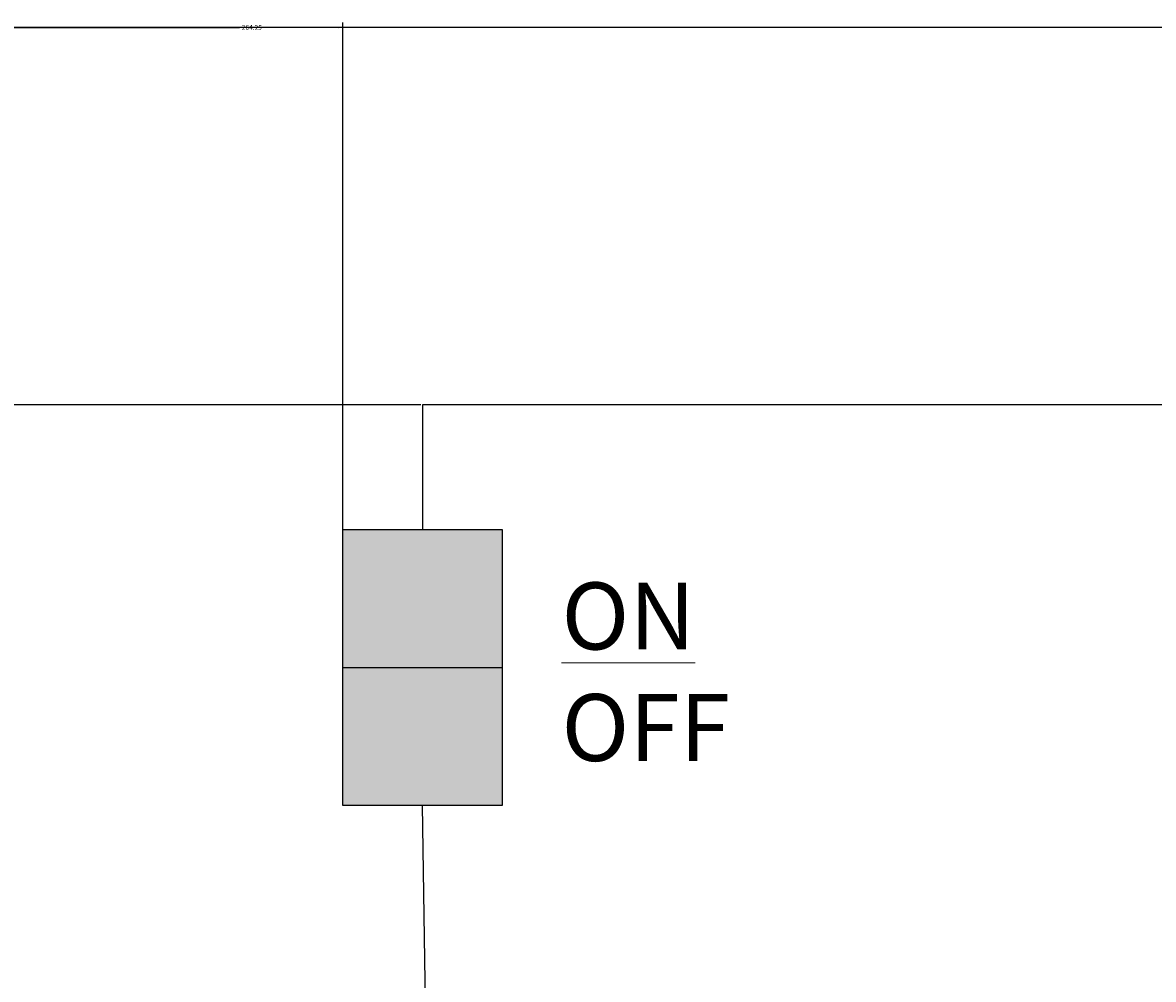
# Model space of a CAD drawing. Units: millimetres. Extents: x -8 to 285, y 5 to 221.
# Tile 25 of 30: x 130 to 172, y 185 to 221. Entities that reach past the tile are written whole.
import ezdxf

# ---------------------------------------------------------------- set-up
doc = ezdxf.new("R2010")
doc.units = ezdxf.units.MM
for name, color, linetype, lineweight in [('A-ANNO-DIMS', 2, 'Continuous', 18), ('E-ANNO-TEXT', 7, 'Continuous', 18), ('E-EQPM-PATT', 252, 'Continuous', 13), ('E-LITE-SWCH', 7, 'Continuous', 25)]:
    doc.layers.add(name, color=color, linetype=linetype, lineweight=lineweight)
doc.layers.add('E-POWR-AC-LINE', color=30, linetype='Continuous', lineweight=25, true_color=0xf26722)
doc.styles.get("Standard").update_dxf_attribs({"font": 'arial.ttf'})
doc.dimstyles.get("Standard").update_dxf_attribs({"dimtxt": 0.18, "dimasz": 0.18, "dimexe": 0.18, "dimexo": 0.0625, "dimgap": 0.09, "dimtad": 0, "dimtih": 1, "dimtoh": 1, "dimdec": 4, "dimzin": 0, "dimdsep": 46, "dimtxsty": 'Standard', "dimcen": 0.09, "dimadec": 0, "dimazin": 0, "dimtfac": 1, "dimtdec": 4, "dimtofl": 0, "dimtmove": 0, "dimatfit": 3, "dimfxl": 1, "dimtolj": 1, "dimtzin": 0, "dimarcsym": 0})

# ---------------------------------------------------------------- blocks, each defined once
blk = doc.blocks.new('SWITCH-ON-OFF')
blk.add_line((0, 5.151), (5.948, 5.151))
blk.add_lwpolyline([(0, 10.303), (5.948, 10.303), (5.948, 0), (0, 0)], close=True)
blk = doc.blocks.new('*D9')
at = {"layer": 'A-ANNO-DIMS', "color": 0, "lineweight": -2, "transparency": 16777216}
for p, q in [((6.672, 133.79), (6.672, 220.737)), ((6.852, 220.557), (138.33, 220.557)), ((270.739, 220.557), (139.262, 220.557)), ((270.919, 206.519), (270.919, 220.737))]:
    blk.add_line(p, q, dxfattribs=at)
at = {"layer": 'A-ANNO-DIMS', "color": 0, "transparency": 16777216}
for points in [[(6.852, 220.587), (6.852, 220.527), (6.672, 220.557)], [(270.739, 220.587), (270.739, 220.527), (270.919, 220.557)]]:
    blk.add_solid(points, dxfattribs=at)
at = {"layer": 'Defpoints', "color": 0, "transparency": 16777216}
for p in [(270.919, 220.557), (270.919, 206.457), (6.672, 133.727)]:
    blk.add_point(p, dxfattribs=at)
at = {"layer": 'A-ANNO-DIMS', "color": 0, "transparency": 16777216, "insert": (138.796, 220.557), "char_height": 0.18, "attachment_point": 5}
blk.add_mtext('\\A1;264.25', dxfattribs=at)
blk = doc.blocks.new('*D10')
at = {"layer": 'A-ANNO-DIMS', "color": 0, "lineweight": -2, "transparency": 16777216}
for p, q in [((145.103, 206.457), (-7.608, 206.457)), ((-7.428, 206.277), (-7.428, 113.161)), ((-7.428, 19.682), (-7.428, 112.797)), ((30.453, 19.502), (-7.608, 19.502))]:
    blk.add_line(p, q, dxfattribs=at)
at = {"layer": 'A-ANNO-DIMS', "color": 0, "transparency": 16777216}
for points in [[(-7.458, 206.277), (-7.398, 206.277), (-7.428, 206.457)], [(-7.458, 19.682), (-7.398, 19.682), (-7.428, 19.502)]]:
    blk.add_solid(points, dxfattribs=at)
at = {"layer": 'Defpoints', "color": 0, "transparency": 16777216}
for p in [(-7.428, 206.457), (145.165, 206.457), (30.516, 19.502)]:
    blk.add_point(p, dxfattribs=at)
at = {"layer": 'A-ANNO-DIMS', "color": 0, "transparency": 16777216, "insert": (-7.428, 112.979), "char_height": 0.18, "attachment_point": 5}
blk.add_mtext('\\A1;186.95', dxfattribs=at)
blk = doc.blocks.new('*D12')
at = {"layer": 'A-ANNO-DIMS', "color": 0, "lineweight": -2, "transparency": 16777216}
for p, q in [((87.572, 192.334), (87.572, 220.737)), ((87.752, 220.557), (114.488, 220.557)), ((142.011, 220.557), (115.274, 220.557)), ((142.191, 191.553), (142.191, 220.737))]:
    blk.add_line(p, q, dxfattribs=at)
at = {"layer": 'A-ANNO-DIMS', "color": 0, "transparency": 16777216}
for points in [[(87.752, 220.587), (87.752, 220.527), (87.572, 220.557)], [(142.011, 220.587), (142.011, 220.527), (142.191, 220.557)]]:
    blk.add_solid(points, dxfattribs=at)
at = {"layer": 'Defpoints', "color": 0, "transparency": 16777216}
for p in [(142.191, 220.557), (87.572, 192.271), (142.191, 191.491)]:
    blk.add_point(p, dxfattribs=at)
at = {"layer": 'A-ANNO-DIMS', "color": 0, "transparency": 16777216, "insert": (114.881, 220.557), "char_height": 0.18, "attachment_point": 5}
blk.add_mtext('\\A1;54.62', dxfattribs=at)

msp = doc.modelspace()

# ---------------------------------------------------------------- hatches: boundary and pattern name
at = {"layer": 'E-EQPM-PATT'}
h = msp.add_hatch(color=256, dxfattribs=at)
h.set_gradient(color2=(0, 0, 0), tint=1)
h.paths.add_polyline_path([(41.1717, 67.9064, 1), (39.1717, 67.9064, 1)])
h.paths.add_polyline_path([(47.1717, 67.9064, 1), (45.1717, 67.9064, 1)])
h.paths.add_polyline_path([(53.1717, 67.9064, 1), (51.1717, 67.9064, 1)])
h.paths.add_polyline_path([(57.1717, 67.9064, 1), (59.1717, 67.9064, 1)])
h.paths.add_polyline_path([(65.1717, 67.9064, 1), (63.1717, 67.9064, 1)])
h.paths.add_polyline_path([(69.1717, 67.9064, 1), (71.1717, 67.9064, 1)])
h.paths.add_polyline_path([(148.1394, 196.6424), (148.1394, 201.7939), (142.1909, 201.7939), (142.1909, 196.6424)])
h.paths.add_polyline_path([(186.1388, 201.7939), (186.1388, 196.6424), (192.0873, 196.6424), (192.0873, 201.7939)])
h.paths.add_polyline_path([(234.0155, 196.6424), (234.0155, 201.7939), (228.067, 201.7939), (228.067, 196.6424)])
h = msp.add_hatch(color=256, dxfattribs=at)
h.set_gradient(color1=(254, 234, 185), color2=(254, 234, 185), tint=1)
h.paths.add_polyline_path([(148.1394, 191.4908), (148.1394, 196.6424), (142.1909, 196.6424), (142.1909, 191.4908)])
h.paths.add_polyline_path([(186.1388, 191.4908), (192.0873, 191.4908), (192.0873, 196.6424), (186.1388, 196.6424)])
h.paths.add_polyline_path([(228.067, 191.4908), (234.0155, 191.4908), (234.0155, 196.6424), (228.067, 196.6424)])

# ---------------------------------------------------------------- linework, layer by layer
at = {"layer": 'E-POWR-AC-LINE'}
msp.add_line((145.2836, 184.1071), (145.1651, 191.4908), dxfattribs=at)
msp.add_lwpolyline([(244.6186, 34.6512), (244.6186, 49.925), (270.9192, 49.925), (270.9192, 206.4568), (145.1651, 206.4568), (145.1651, 201.7939)], dxfattribs=at)

# ---------------------------------------------------------------- block references
at = {"layer": 'E-LITE-SWCH'}
msp.add_blockref('SWITCH-ON-OFF', (142.191, 191.491), dxfattribs=at)

# ---------------------------------------------------------------- texts
at = {"layer": 'E-ANNO-TEXT', "insert": (149.5968, 199.8179), "char_height": 2.5, "attachment_point": 1}
msp.add_mtext_dynamic_manual_height_columns(' {\\LON\\P} OFF', width=8.619646, gutter_width=12.5, heights=[7.2553], dxfattribs=at)

# ---------------------------------------------------------------- dimensions: what is measured, and where the dimension line sits
at = {"layer": 'A-ANNO-DIMS'}
for base, p1, p2, picture, middle in [((270.9192, 220.5568), (6.6725, 133.7273), (270.9192, 206.4568), '*D9', (138.7958, 220.5568)), ((142.1909, 220.5568), (87.5716, 192.2715), (142.1909, 191.4908), '*D12', (114.8812, 220.5568))]:
    dim = msp.add_linear_dim(base=base, p1=p1, p2=p2, dimstyle='Standard', override={"dimdec": 2, "dimlfac": 1, "dimrnd": 0, "dimzin": 0, "dimdsep": 46, "dimlunit": 2}, dxfattribs=at)
    dim.commit()
    dim.dimension.update_dxf_attribs({"geometry": picture, "text_midpoint": middle})
dim = msp.add_linear_dim(base=(-7.4275, 206.4568), p1=(30.516, 19.502), p2=(145.1651, 206.4568), angle=90, dimstyle='Standard', override={"dimdec": 2, "dimlfac": 1, "dimrnd": 0, "dimzin": 0, "dimdsep": 46, "dimlunit": 2}, dxfattribs=at)
dim.commit()
dim.dimension.update_dxf_attribs({"geometry": '*D10', "text_midpoint": (-7.4275, 112.9794)})

doc.saveas('drawing.dxf')
